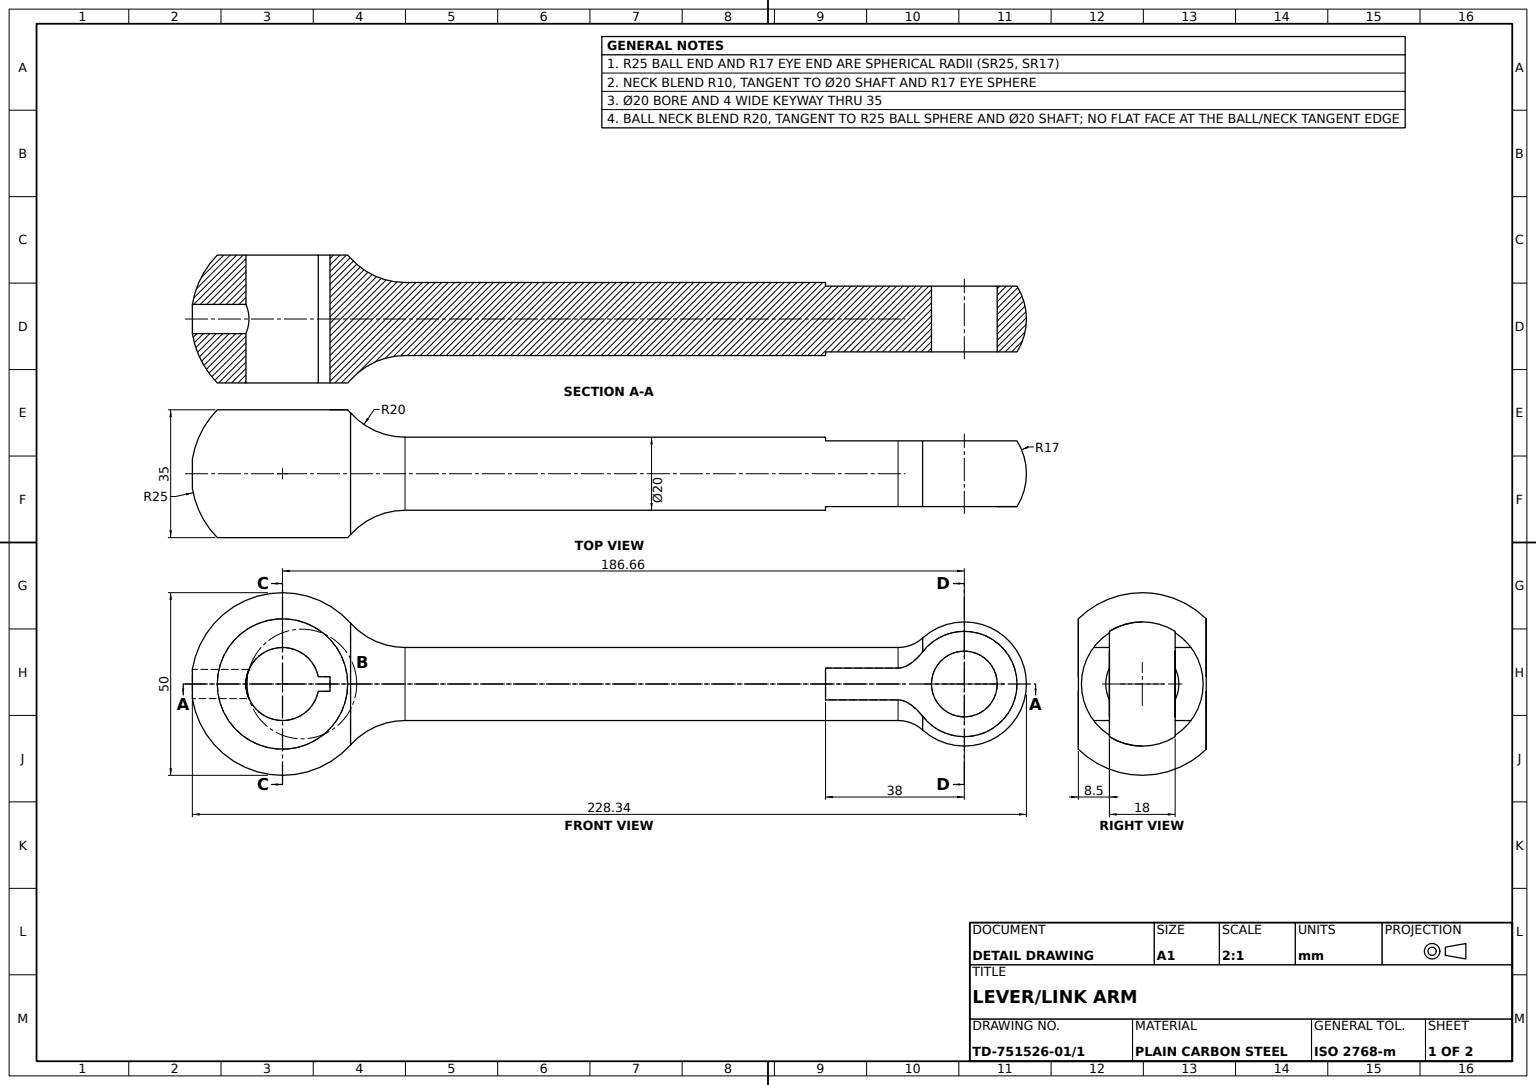
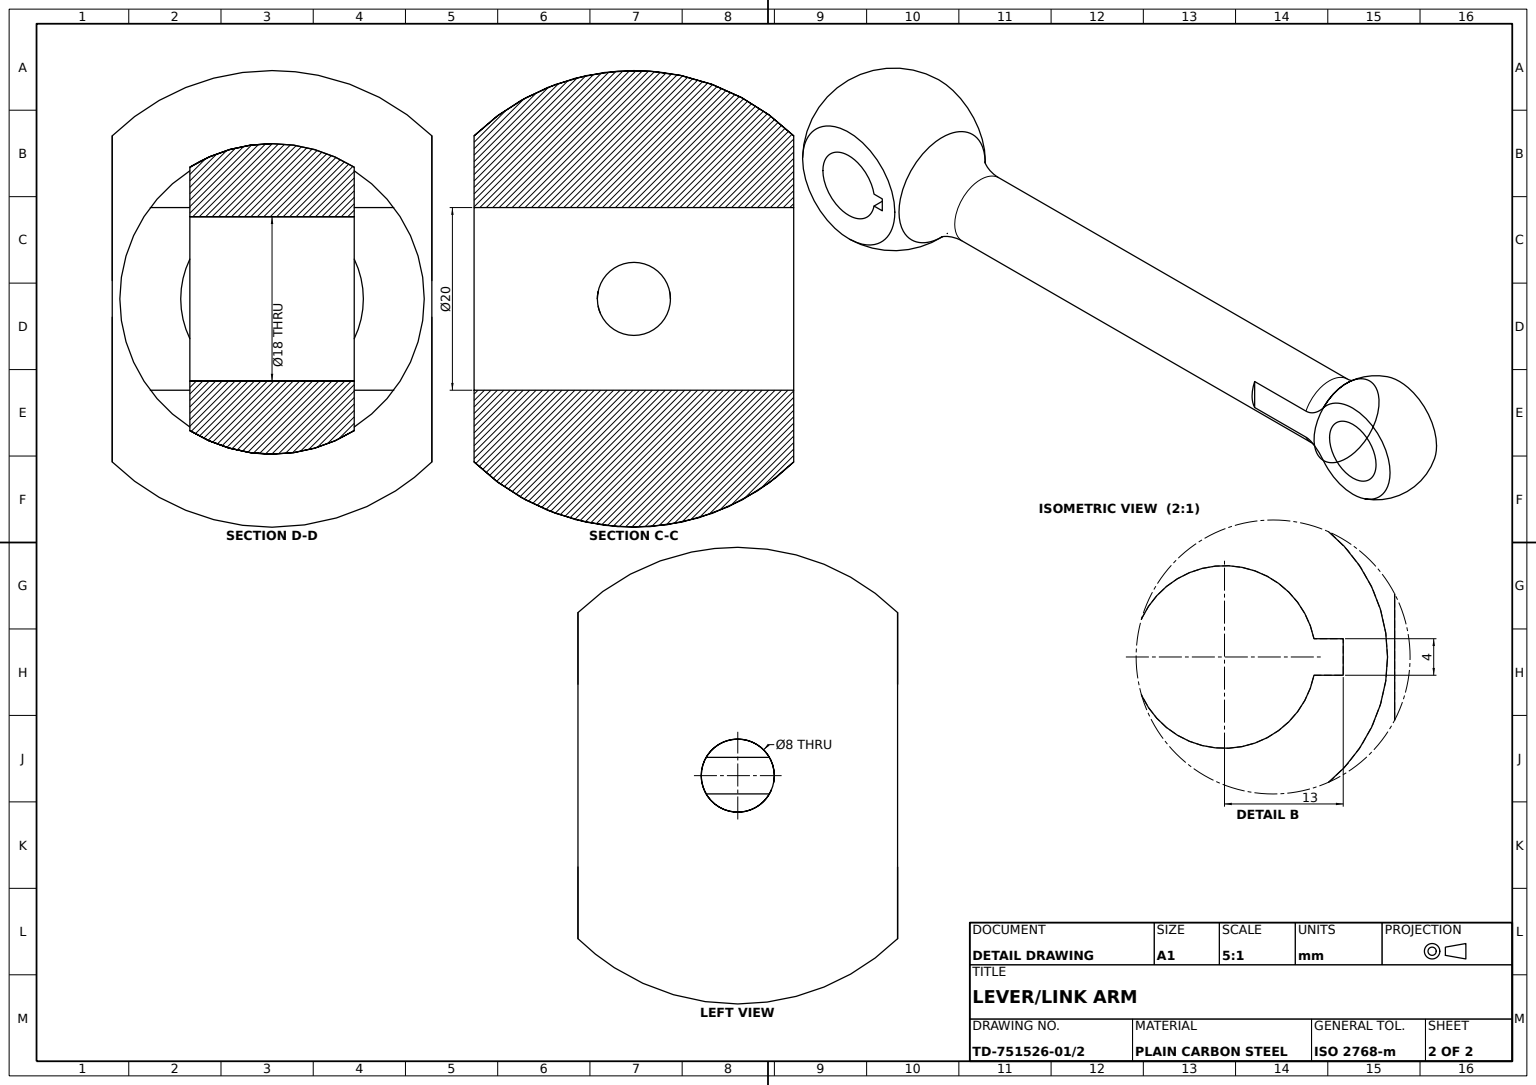
from build123d import *

# Parameters (mm, degrees)
BALL_FACE_1_SKETCH_R       = 25
BALL_FACE_CUT_1_DEPTH      = 7.5
BALL_FACE_2_SKETCH_R       = 25
BALL_FACE_CUT_2_DEPTH      = 7.5
KEYED_BORE_20_REACH        = 210.153
SMALL_END_FLAT_CUT_1_REACH = 216.934
SMALL_START                = -9
SMALL_END_FLAT_CUT_2_REACH = 216.934
SMALL_START_2              = 9
SMALL_END_EYE_CUT_REACH    = 208.893
SMALL_END_EYE_SKETCH_R     = 9
HOLE_8_CUT_REACH           = 207.934
HOLE_8_CUT_END_RADIUS      = 25
HOLE_8_SKETCH_R            = 4


with BuildPart() as part:
    # Lever Profile Sketch → Lever Body Revolve (revolve)
    with BuildSketch(Plane(origin=(0, 0, 0), x_dir=(1, 0, 0), z_dir=(0, 1, 0)), mode=Mode.PRIVATE) as lever_body_revolve_sk:
        with BuildLine():
            Line((168.522248412, -10), (33.541019662, -10))
            ThreePointArc((33.541019662, -10), (25.376053853, -11.742581416), (18.633899812, -16.666666667))
            ThreePointArc((18.633899812, -16.666666667), (-8.920552244, -23.354308974), (-25, 0))
            Line((-25, 0), (203.66060556, 0))
            ThreePointArc((203.66060556, 0), (193.547273819, -15.542644572), (175.240158467, -12.592592593))
            ThreePointArc((175.240158467, -12.592592593), (172.122659912, -10.670635765), (168.522248412, -10))
        make_face()
    revolve(lever_body_revolve_sk.sketch.rotate(Axis((248.139692176, 0, 0), (-1, 0, 0)), 180), axis=Axis((248.139692176, 0, 0), (-1, 0, 0)))

    # Ball Face 1 Sketch → Ball Face Cut 1 (cut)
    with BuildSketch(Plane.XY.offset(25)):
        Circle(BALL_FACE_1_SKETCH_R)
    extrude(amount=-BALL_FACE_CUT_1_DEPTH, mode=Mode.SUBTRACT)


with BuildPart() as ball_face_cut_1_kept_piece:
    # of the separate pieces the step leaves, the one the design keeps (ball_face_cut_1_pieces_kept)
    add(part.part.solids().sort_by_distance((175.240158467, 0, -12.592592593))[0])

    # Ball Face 2 Sketch → Ball Face Cut 2 (cut)
    with BuildSketch(Plane.XY.offset(-25)):
        Circle(BALL_FACE_2_SKETCH_R)
    extrude(amount=BALL_FACE_CUT_2_DEPTH, mode=Mode.SUBTRACT)

    # Keyed Bore Sketch → Keyed Bore _20 (cut, up to next)
    with BuildSketch(Plane(origin=(0, 0, -17.5), x_dir=(-1, 0, 0), z_dir=(0, 0, -1)), mode=Mode.PRIVATE) as keyed_bore_20_sk1:
        with BuildLine():
            Line((-13, 2), (-9.797958971, 2))
            ThreePointArc((-9.797958971, 2), (10, 0), (-9.797958971, -2))
            Line((-9.797958971, -2), (-13, -2))
            Line((-13, -2), (-13, 2))
        make_face()
    keyed_bore_20_tool1 = extrude(keyed_bore_20_sk1.sketch, amount=-KEYED_BORE_20_REACH, mode=Mode.PRIVATE) & ball_face_cut_1_kept_piece.part
    add(keyed_bore_20_tool1.solids().sort_by_distance((0.430928, 0, -17.5))[0], mode=Mode.SUBTRACT)

    # Small End Flats Sketch → Small End Flat Cut 1 (cut, up to next)
    with BuildSketch(Plane.XY.offset(SMALL_START), mode=Mode.PRIVATE) as small_end_flat_cut_1_sk1:
        with BuildLine():
            Line((170.41252875, 5), (148.66060556, 5))
            Line((148.66060556, 5), (148.66060556, -5))
            Line((148.66060556, -5), (170.41252875, -5))
            ThreePointArc((170.41252875, -5), (203.66060556, 0), (170.41252875, 5))
        make_face()
    small_end_flat_cut_1_tool1 = extrude(small_end_flat_cut_1_sk1.sketch, amount=-SMALL_END_FLAT_CUT_1_REACH, mode=Mode.PRIVATE) & ball_face_cut_1_kept_piece.part
    add(small_end_flat_cut_1_tool1.solids().sort_by_distance((181.469026, 0, -9))[0], mode=Mode.SUBTRACT)

    # Sketch11_2 → Small End Flat Cut 2 (cut, up to next)
    with BuildSketch(Plane.XY.offset(SMALL_START_2), mode=Mode.PRIVATE) as small_end_flat_cut_2_sk1:
        with BuildLine():
            Line((170.41252875, 5), (148.66060556, 5))
            Line((148.66060556, 5), (148.66060556, -5))
            Line((148.66060556, -5), (170.41252875, -5))
            ThreePointArc((170.41252875, -5), (203.66060556, 0), (170.41252875, 5))
        make_face()
    small_end_flat_cut_2_tool1 = extrude(small_end_flat_cut_2_sk1.sketch, amount=SMALL_END_FLAT_CUT_2_REACH, mode=Mode.PRIVATE) & ball_face_cut_1_kept_piece.part
    add(small_end_flat_cut_2_tool1.solids().sort_by_distance((181.469026, 0, 9))[0], mode=Mode.SUBTRACT)

    # Small End Eye Sketch → Small End Eye Cut (cut, up to next)
    with BuildSketch(Plane.XY.offset(9), mode=Mode.PRIVATE) as small_end_eye_cut_sk1:
        with Locations((186.66060556, 0)):
            Circle(SMALL_END_EYE_SKETCH_R)
    small_end_eye_cut_tool1 = extrude(small_end_eye_cut_sk1.sketch, amount=-SMALL_END_EYE_CUT_REACH, mode=Mode.PRIVATE) & ball_face_cut_1_kept_piece.part
    add(small_end_eye_cut_tool1.solids().sort_by_distance((186.660606, 0, 9))[0], mode=Mode.SUBTRACT)

    # Hole _8 Cut: up to this sphere (the profile starts inside it)
    hole_8_cut_end = Location((0, 0, 0)) * Sphere(HOLE_8_CUT_END_RADIUS, mode=Mode.PRIVATE)
    # Hole _8 Sketch → Hole _8 Cut (cut, up to the surface)
    with BuildSketch(Plane(origin=(0, 0, 0), x_dir=(0, 0, -1), z_dir=(1, 0, 0)), mode=Mode.PRIVATE) as hole_8_cut_sk1:
        Circle(HOLE_8_SKETCH_R)
    hole_8_cut_tool1 = extrude(hole_8_cut_sk1.sketch, amount=-HOLE_8_CUT_REACH, mode=Mode.PRIVATE) & hole_8_cut_end
    add(hole_8_cut_tool1.solids().sort_by_distance((0, 0, 0))[0], mode=Mode.SUBTRACT)


solid = ball_face_cut_1_kept_piece.part
